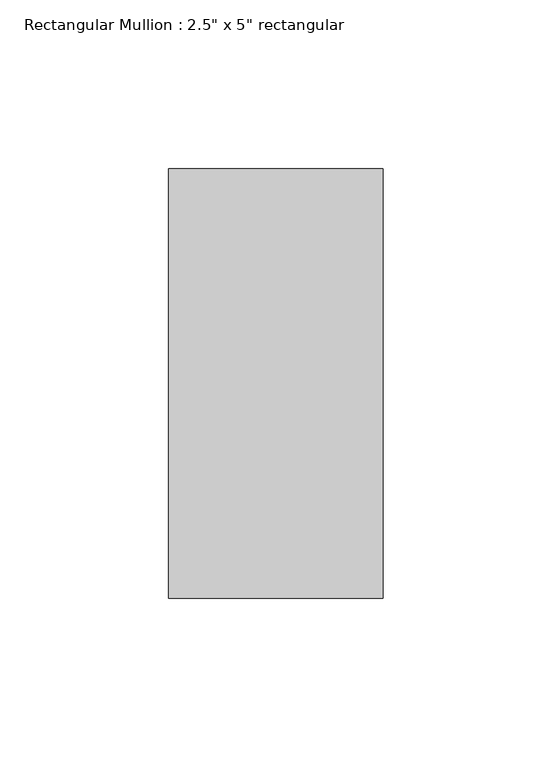
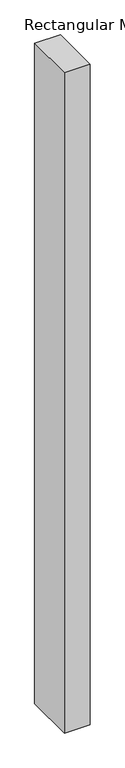
"""IFC4 building model written with IfcOpenShell, lengths in millimetres: member geometry."""

from ifc_helpers import new_model, si_unit, frame, origin, place, context, project, spatial, polyline, outline, extrude, source, transform, mapped, element, save


def member_e59d77c9(model_context):
    return source(origin(), model_context, "Body", "SweptSolid", [
        extrude(outline(polyline([(31.75, 63.5), (31.75, -63.5), (-31.75, -63.5), (-31.75, 63.5), (31.75, 63.5)])), frame((0.0, 0.0, -1720.7849865), z_axis=(0.0, 0.0, 1.0), x_axis=(1.0, 0.0, 0.0)), (0.0, 0.0, 1.0), 1720.7849865),
    ])


if __name__ == "__main__":
    model = new_model("IFC4")
    model_context = context("Model", 3, world=origin())
    ifc_project = project(units=[si_unit("LENGTHUNIT", "METRE", prefix="MILLI")], contexts=[model_context])
    site = spatial("IfcSite", under=ifc_project)
    building = spatial("IfcBuilding", under=site)
    placement = place(None, origin())
    member_shape = member_e59d77c9(model_context)
    element("IfcMember", 1, ObjectType="Rectangular Mullion : 2.5\" x 5\" rectangular", at=placement, inside=building, context=model_context, shape_type="MappedRepresentation", body=[
        mapped(member_shape, transform((0.0, 0.0, 0.0), x_axis=(1.0, 0.0, 0.0), y_axis=(0.0, 1.0, 0.0), z_axis=(0.0, 0.0, 1.0))),
    ])
    save(model, "model.ifc")

# Revit data of these elements
# Type "Rectangular Mullion : 2.5\" x 5\" rectangular"
#   built-in parameter 1007304 = 0.416667 (stored number, unit not read)
#   built-in parameter 1007301 = 0.104167 (stored number, unit not read)
#   built-in parameter 1007300 = 0.104167 (stored number, unit not read)
# Element 1 (IfcMember, "Rectangular Mullion : 2.5\" x 5\" rectangular")
#   Materials on its faces: "Aluminum"
# Materials
#   "Aluminum": class "Metal", colour RGB 247 247 247, transparency 0, Description = "Aluminum 6061", Cost = 0
